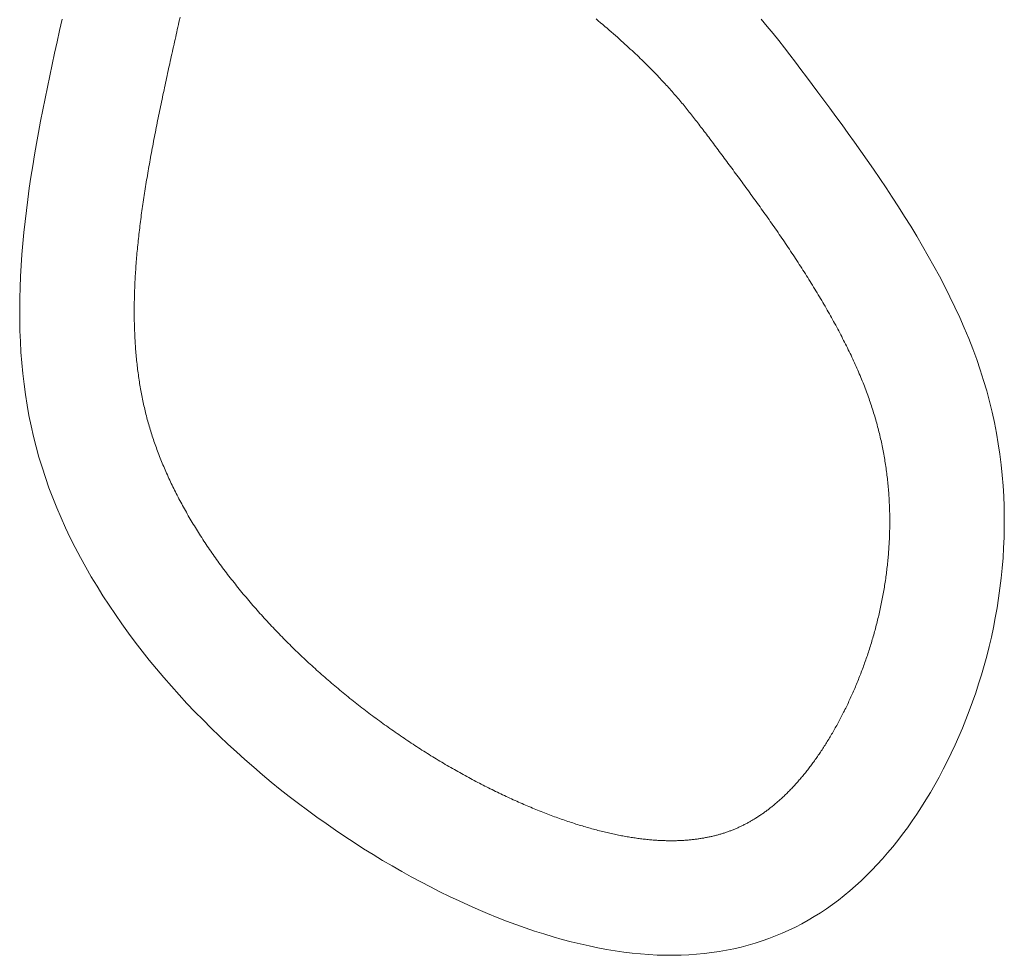
# Model space of a CAD drawing. Units: inches. Extents: x 64 to 1167, y 117 to 939.
# Tile 15 of 56: x 193.497 to 197.794, y 849.033 to 853.116. Entities that reach past the tile are written whole.
import ezdxf

# ---------------------------------------------------------------- set-up
doc = ezdxf.new("R2010")
doc.units = ezdxf.units.IN
doc.header["$MEASUREMENT"] = 0
doc.layers.add('A-FLOR-FIXT', color=8, linetype='Continuous', lineweight=18)

# ---------------------------------------------------------------- blocks, each defined once
blk = doc.blocks.new('FAUCET')
for points in [[(4.0816, 3.6354, 0), (4.1129, 3.6621, 0), (4.144, 3.6879, 0), (4.175, 3.713, 0), (4.2059, 3.7375, 0), (4.2371, 3.7616, 0), (4.2685, 3.7856, 0), (4.3004, 3.8096, 0), (4.3329, 3.8338, 0), (4.366, 3.8585, 0), (4.3999, 3.8837, 0), (4.4345, 3.9094, 0), (4.4699, 3.9356, 0), (4.506, 3.9621, 0), (4.5427, 3.989, 0), (4.5802, 4.0161, 0), (4.6182, 4.0434, 0), (4.6569, 4.0709, 0), (4.6961, 4.0984, 0), (4.7359, 4.126, 0), (4.7762, 4.1535, 0), (4.817, 4.181, 0), (4.8584, 4.2082, 0), (4.9002, 4.2353, 0), (4.9424, 4.2621, 0), (4.985, 4.2886, 0), (5.0281, 4.3147, 0), (5.0715, 4.3404, 0), (5.1152, 4.3655, 0), (5.1593, 4.3901, 0), (5.2036, 4.4141, 0), (5.2483, 4.4374, 0), (5.2931, 4.46, 0), (5.3382, 4.4817, 0), (5.3835, 4.5026, 0), (5.429, 4.5226, 0), (5.4746, 4.5416, 0), (5.5203, 4.5596, 0), (5.5662, 4.5765, 0), (5.6121, 4.5923, 0), (5.6581, 4.6068, 0), (5.7041, 4.6202, 0), (5.7502, 4.6325, 0), (5.7962, 4.6436, 0), (5.8423, 4.6537, 0), (5.8883, 4.6626, 0), (5.9343, 4.6705, 0), (5.9802, 4.6773, 0), (6.0261, 4.6831, 0), (6.0718, 4.6878, 0), (6.1175, 4.6916, 0), (6.163, 4.6944, 0), (6.2084, 4.6962, 0), (6.2536, 4.697, 0), (6.2986, 4.697, 0), (6.3435, 4.696, 0), (6.3882, 4.6942, 0), (6.4326, 4.6915, 0), (6.4768, 4.6879, 0), (6.5207, 4.6835, 0), (6.5644, 4.6782, 0), (6.6078, 4.6722, 0), (6.6509, 4.6654, 0), (6.6936, 4.6578, 0), (6.736, 4.6495, 0), (6.7781, 4.6405, 0), (6.8198, 4.6308, 0), (6.8611, 4.6203, 0), (6.902, 4.6092, 0), (6.9425, 4.5975, 0), (6.9825, 4.5851, 0), (7.0221, 4.5721, 0), (7.0612, 4.5585, 0), (7.0999, 4.5443, 0), (7.138, 4.5295, 0), (7.1756, 4.5143, 0), (7.2127, 4.4985, 0), (7.2492, 4.4821, 0), (7.2852, 4.4653, 0), (7.3206, 4.4481, 0), (7.3553, 4.4303, 0), (7.3895, 4.4122, 0), (7.423, 4.3936, 0), (7.4559, 4.3746, 0), (7.4881, 4.3553, 0), (7.5196, 4.3356, 0), (7.5504, 4.3155, 0), (7.5806, 4.2951, 0), (7.61, 4.2744, 0), (7.6387, 4.2533, 0), (7.6666, 4.2319, 0), (7.6939, 4.2101, 0), (7.7205, 4.188, 0), (7.7463, 4.1655, 0), (7.7714, 4.1426, 0), (7.7957, 4.1195, 0), (7.8193, 4.0959, 0), (7.8422, 4.072, 0), (7.8643, 4.0478, 0), (7.8857, 4.0231, 0), (7.9064, 3.9982, 0), (7.9262, 3.9728, 0), (7.9454, 3.9471, 0), (7.9637, 3.921, 0), (7.9813, 3.8946, 0), (7.9981, 3.8678, 0), (8.0142, 3.8406, 0), (8.0294, 3.8131, 0), (8.0439, 3.7852, 0), (8.0576, 3.7569, 0), (8.0705, 3.7282, 0), (8.0827, 3.6991, 0), (8.094, 3.6697, 0), (8.1045, 3.6399, 0), (8.1142, 3.6097, 0), (8.1231, 3.5791, 0), (8.1312, 3.5482, 0), (8.1385, 3.5168, 0), (8.145, 3.4851, 0), (8.1507, 3.453, 0), (8.1555, 3.4204, 0), (8.1595, 3.3875, 0), (8.1626, 3.3542, 0), (8.165, 3.3205, 0), (8.1665, 3.2864, 0), (8.1671, 3.252, 0), (8.1669, 3.2171, 0), (8.1659, 3.1818, 0), (8.164, 3.1461, 0), (8.1612, 3.11, 0), (8.1576, 3.0735, 0), (8.1531, 3.0366, 0), (8.1477, 2.9992, 0), (8.1415, 2.9615, 0), (8.1344, 2.9234, 0), (8.1264, 2.8849, 0), (8.1176, 2.846, 0), (8.108, 2.8068, 0), (8.0975, 2.7673, 0), (8.0862, 2.7275, 0), (8.074, 2.6874, 0), (8.0611, 2.647, 0), (8.0474, 2.6065, 0), (8.0329, 2.5657, 0), (8.0176, 2.5247, 0), (8.0016, 2.4835, 0), (7.9848, 2.4422, 0), (7.9672, 2.4008, 0), (7.9489, 2.3592, 0), (7.9299, 2.3176, 0), (7.9102, 2.2759, 0), (7.8898, 2.2341, 0), (7.8686, 2.1924, 0), (7.8468, 2.1506, 0), (7.8243, 2.1088, 0), (7.8011, 2.0671, 0), (7.7772, 2.0254, 0), (7.7527, 1.9838, 0), (7.7276, 1.9423, 0), (7.7018, 1.9009, 0), (7.6754, 1.8597, 0), (7.6484, 1.8186, 0), (7.6207, 1.7777, 0), (7.5925, 1.737, 0), (7.5637, 1.6965, 0), (7.5343, 1.6563, 0), (7.5043, 1.6163, 0), (7.4738, 1.5766, 0), (7.4428, 1.5372, 0), (7.4112, 1.4981, 0), (7.379, 1.4594, 0), (7.3464, 1.4211, 0), (7.3132, 1.3831, 0), (7.2795, 1.3456, 0), (7.2453, 1.3085, 0), (7.2107, 1.2718, 0), (7.1755, 1.2356, 0), (7.1399, 1.1999, 0), (7.1039, 1.1647, 0), (7.0674, 1.13, 0), (7.0305, 1.0959, 0), (6.9931, 1.0624, 0), (6.9553, 1.0294, 0), (6.9171, 0.9971, 0), (6.8785, 0.9654, 0), (6.8396, 0.9344, 0), (6.8002, 0.904, 0), (6.7605, 0.8744, 0), (6.7204, 0.8455, 0), (6.6799, 0.8173, 0), (6.6391, 0.7898, 0), (6.598, 0.7632, 0), (6.5566, 0.7373, 0), (6.5148, 0.7123, 0), (6.4727, 0.6881, 0), (6.4304, 0.6648, 0), (6.3877, 0.6424, 0), (6.3448, 0.6208, 0), (6.3016, 0.6002, 0), (6.2581, 0.5806, 0), (6.2144, 0.5619, 0), (6.1705, 0.5442, 0), (6.1263, 0.5275, 0), (6.0819, 0.5119, 0), (6.0373, 0.4973, 0), (5.9925, 0.4837, 0), (5.9475, 0.4713, 0), (5.9023, 0.4599, 0), (5.8569, 0.4497, 0), (5.8114, 0.4404, 0), (5.7657, 0.4322, 0), (5.7198, 0.425, 0), (5.6737, 0.4187, 0), (5.6275, 0.4134, 0), (5.5811, 0.409, 0), (5.5345, 0.4055, 0), (5.4878, 0.4029, 0), (5.441, 0.401, 0), (5.394, 0.4, 0), (5.3468, 0.3998, 0), (5.2995, 0.4004, 0), (5.2521, 0.4017, 0), (5.2045, 0.4036, 0), (5.1568, 0.4063, 0), (5.109, 0.4096, 0), (5.0611, 0.4136, 0), (5.013, 0.4182, 0), (4.9648, 0.4233, 0), (4.9165, 0.429, 0), (4.8681, 0.4352, 0), (4.8196, 0.4419, 0), (4.771, 0.4491, 0), (4.7222, 0.4568, 0), (4.6734, 0.4648, 0), (4.6245, 0.4733, 0), (4.5755, 0.4822, 0), (4.5264, 0.4913, 0), (4.4772, 0.5008, 0), (4.428, 0.5106, 0), (4.3786, 0.5207, 0), (4.3292, 0.531, 0), (4.2798, 0.5415, 0), (4.2302, 0.5522, 0), (4.1806, 0.5631, 0), (4.131, 0.5741, 0), (4.0812, 0.5853, 0)], [(4.0798, 2.9151, 0), (4.0883, 2.9251, 0), (4.0967, 2.935, 0), (4.1049, 2.9447, 0), (4.1131, 2.9542, 0), (4.1212, 2.9636, 0), (4.1292, 2.9729, 0), (4.1371, 2.9819, 0), (4.145, 2.9909, 0), (4.1527, 2.9996, 0), (4.1603, 3.0083, 0), (4.1679, 3.0168, 0), (4.1754, 3.0251, 0), (4.1828, 3.0333, 0), (4.1901, 3.0414, 0), (4.1973, 3.0493, 0), (4.2045, 3.0572, 0), (4.2116, 3.0648, 0), (4.2186, 3.0724, 0), (4.2256, 3.0798, 0), (4.2324, 3.0871, 0), (4.2392, 3.0943, 0), (4.246, 3.1013, 0), (4.2526, 3.1083, 0), (4.2592, 3.1151, 0), (4.2658, 3.1219, 0), (4.2722, 3.1285, 0), (4.2786, 3.135, 0), (4.285, 3.1414, 0), (4.2913, 3.1477, 0), (4.2975, 3.1539, 0), (4.3037, 3.16, 0), (4.3098, 3.166, 0), (4.3159, 3.1719, 0), (4.3219, 3.1777, 0), (4.3279, 3.1835, 0), (4.3338, 3.1891, 0), (4.3397, 3.1947, 0), (4.3456, 3.2002, 0), (4.3514, 3.2057, 0), (4.3572, 3.211, 0), (4.3629, 3.2164, 0), (4.3687, 3.2216, 0), (4.3744, 3.2268, 0), (4.3801, 3.2319, 0), (4.3857, 3.237, 0), (4.3914, 3.242, 0), (4.397, 3.247, 0), (4.4026, 3.252, 0), (4.4082, 3.2569, 0), (4.4138, 3.2617, 0), (4.4194, 3.2665, 0), (4.425, 3.2713, 0), (4.4306, 3.2761, 0), (4.4362, 3.2808, 0), (4.4418, 3.2855, 0), (4.4474, 3.2902, 0), (4.453, 3.2948, 0), (4.4587, 3.2995, 0), (4.4643, 3.3041, 0), (4.47, 3.3087, 0), (4.4756, 3.3133, 0), (4.4813, 3.3179, 0), (4.4871, 3.3224, 0), (4.4928, 3.327, 0), (4.4986, 3.3316, 0), (4.5044, 3.3362, 0), (4.5103, 3.3408, 0), (4.5161, 3.3454, 0), (4.5221, 3.35, 0), (4.528, 3.3546, 0), (4.534, 3.3592, 0), (4.5401, 3.3639, 0), (4.5462, 3.3685, 0), (4.5523, 3.3732, 0), (4.5585, 3.378, 0), (4.5648, 3.3827, 0), (4.5711, 3.3875, 0), (4.5775, 3.3923, 0), (4.5839, 3.3972, 0), (4.5905, 3.4021, 0), (4.597, 3.407, 0), (4.6037, 3.412, 0), (4.6104, 3.417, 0), (4.6172, 3.4221, 0), (4.624, 3.4272, 0), (4.6309, 3.4324, 0), (4.6379, 3.4376, 0), (4.6448, 3.4428, 0), (4.6519, 3.448, 0), (4.659, 3.4533, 0), (4.6661, 3.4586, 0), (4.6733, 3.464, 0), (4.6805, 3.4694, 0), (4.6877, 3.4748, 0), (4.695, 3.4802, 0), (4.7024, 3.4856, 0), (4.7097, 3.4911, 0), (4.7171, 3.4966, 0), (4.7246, 3.5021, 0), (4.732, 3.5076, 0), (4.7395, 3.5132, 0), (4.747, 3.5187, 0), (4.7546, 3.5243, 0), (4.7621, 3.5299, 0), (4.7697, 3.5355, 0), (4.7773, 3.541, 0), (4.7849, 3.5466, 0), (4.7926, 3.5523, 0), (4.8002, 3.5579, 0), (4.8079, 3.5635, 0), (4.8156, 3.5691, 0), (4.8232, 3.5747, 0), (4.8309, 3.5803, 0), (4.8386, 3.5859, 0), (4.8464, 3.5915, 0), (4.8541, 3.5972, 0), (4.8619, 3.6028, 0), (4.8696, 3.6084, 0), (4.8774, 3.614, 0), (4.8852, 3.6196, 0), (4.8931, 3.6253, 0), (4.9009, 3.6309, 0), (4.9088, 3.6365, 0), (4.9167, 3.6421, 0), (4.9246, 3.6478, 0), (4.9325, 3.6534, 0), (4.9404, 3.659, 0), (4.9484, 3.6646, 0), (4.9563, 3.6702, 0), (4.9643, 3.6758, 0), (4.9723, 3.6814, 0), (4.9803, 3.687, 0), (4.9883, 3.6926, 0), (4.9964, 3.6982, 0), (5.0044, 3.7038, 0), (5.0125, 3.7094, 0), (5.0206, 3.7149, 0), (5.0286, 3.7205, 0), (5.0367, 3.726, 0), (5.0449, 3.7316, 0), (5.053, 3.7371, 0), (5.0611, 3.7426, 0), (5.0693, 3.7481, 0), (5.0774, 3.7536, 0), (5.0856, 3.7591, 0), (5.0938, 3.7645, 0), (5.102, 3.77, 0), (5.1102, 3.7754, 0), (5.1184, 3.7808, 0), (5.1266, 3.7862, 0), (5.1349, 3.7916, 0), (5.1431, 3.797, 0), (5.1514, 3.8023, 0), (5.1596, 3.8077, 0), (5.1679, 3.813, 0), (5.1762, 3.8183, 0), (5.1844, 3.8235, 0), (5.1927, 3.8288, 0), (5.201, 3.834, 0), (5.2093, 3.8393, 0), (5.2176, 3.8444, 0), (5.2259, 3.8496, 0), (5.2342, 3.8548, 0), (5.2425, 3.8599, 0), (5.2509, 3.865, 0), (5.2592, 3.8701, 0), (5.2675, 3.8751, 0), (5.2758, 3.8801, 0), (5.2841, 3.8851, 0), (5.2925, 3.8901, 0), (5.3008, 3.8951, 0), (5.3091, 3.9, 0), (5.3174, 3.9049, 0), (5.3258, 3.9097, 0), (5.3341, 3.9146, 0), (5.3424, 3.9194, 0), (5.3507, 3.9241, 0), (5.359, 3.9289, 0), (5.3673, 3.9336, 0), (5.3757, 3.9382, 0), (5.384, 3.9429, 0), (5.3923, 3.9475, 0), (5.4005, 3.9521, 0), (5.4088, 3.9566, 0), (5.4171, 3.9611, 0), (5.4254, 3.9656, 0), (5.4337, 3.97, 0), (5.4419, 3.9744, 0), (5.4502, 3.9788, 0), (5.4584, 3.9831, 0), (5.4667, 3.9874, 0), (5.4749, 3.9916, 0), (5.4831, 3.9959, 0), (5.4913, 4, 0), (5.4995, 4.0042, 0), (5.5077, 4.0082, 0), (5.5159, 4.0123, 0), (5.5241, 4.0163, 0), (5.5322, 4.0203, 0), (5.5403, 4.0242, 0), (5.5485, 4.028, 0), (5.5566, 4.0319, 0), (5.5647, 4.0357, 0), (5.5728, 4.0394, 0), (5.5808, 4.0431, 0), (5.5889, 4.0467, 0), (5.5969, 4.0503, 0), (5.6049, 4.0539, 0), (5.6129, 4.0574, 0), (5.6209, 4.0608, 0), (5.6288, 4.0642, 0), (5.6367, 4.0676, 0), (5.6446, 4.0708, 0), (5.6525, 4.0741, 0), (5.6604, 4.0773, 0), (5.6682, 4.0804, 0), (5.676, 4.0835, 0), (5.6838, 4.0866, 0), (5.6916, 4.0896, 0), (5.6994, 4.0926, 0), (5.7072, 4.0955, 0), (5.7149, 4.0983, 0), (5.7226, 4.1012, 0), (5.7304, 4.1039, 0), (5.7381, 4.1067, 0), (5.7457, 4.1093, 0), (5.7534, 4.112, 0), (5.7611, 4.1146, 0), (5.7687, 4.1171, 0), (5.7764, 4.1196, 0), (5.784, 4.1221, 0), (5.7916, 4.1245, 0), (5.7992, 4.1269, 0), (5.8069, 4.1292, 0), (5.8144, 4.1315, 0), (5.822, 4.1337, 0), (5.8296, 4.1359, 0), (5.8372, 4.1381, 0), (5.8448, 4.1402, 0), (5.8523, 4.1422, 0), (5.8599, 4.1443, 0), (5.8674, 4.1462, 0), (5.875, 4.1482, 0), (5.8825, 4.1501, 0), (5.89, 4.1519, 0), (5.8976, 4.1538, 0), (5.9051, 4.1555, 0), (5.9126, 4.1573, 0), (5.9202, 4.159, 0), (5.9277, 4.1606, 0), (5.9352, 4.1623, 0), (5.9428, 4.1638, 0), (5.9503, 4.1654, 0), (5.9578, 4.1669, 0), (5.9654, 4.1683, 0), (5.9729, 4.1698, 0), (5.9804, 4.1712, 0), (5.988, 4.1725, 0), (5.9955, 4.1738, 0), (6.0031, 4.1751, 0), (6.0106, 4.1763, 0), (6.0182, 4.1775, 0), (6.0257, 4.1787, 0), (6.0333, 4.1798, 0), (6.0409, 4.1809, 0), (6.0485, 4.182, 0), (6.056, 4.183, 0), (6.0636, 4.184, 0), (6.0712, 4.1849, 0), (6.0788, 4.1858, 0), (6.0864, 4.1867, 0), (6.094, 4.1875, 0), (6.1016, 4.1883, 0), (6.1092, 4.1891, 0), (6.1168, 4.1898, 0), (6.1244, 4.1905, 0), (6.132, 4.1912, 0), (6.1396, 4.1918, 0), (6.1472, 4.1924, 0), (6.1548, 4.193, 0), (6.1624, 4.1935, 0), (6.17, 4.194, 0), (6.1776, 4.1944, 0), (6.1852, 4.1948, 0), (6.1928, 4.1952, 0), (6.2004, 4.1956, 0), (6.208, 4.1959, 0), (6.2155, 4.1961, 0), (6.2231, 4.1964, 0), (6.2307, 4.1966, 0), (6.2383, 4.1968, 0), (6.2459, 4.1969, 0), (6.2534, 4.197, 0), (6.261, 4.1971, 0), (6.2686, 4.1971, 0), (6.2761, 4.1971, 0), (6.2837, 4.1971, 0), (6.2913, 4.197, 0), (6.2988, 4.1969, 0), (6.3064, 4.1968, 0), (6.3139, 4.1967, 0), (6.3215, 4.1965, 0), (6.329, 4.1962, 0), (6.3365, 4.196, 0), (6.3441, 4.1957, 0), (6.3516, 4.1954, 0), (6.3591, 4.195, 0), (6.3666, 4.1946, 0), (6.3741, 4.1942, 0), (6.3817, 4.1937, 0), (6.3892, 4.1933, 0), (6.3967, 4.1927, 0), (6.4042, 4.1922, 0), (6.4116, 4.1916, 0), (6.4191, 4.191, 0), (6.4266, 4.1904, 0), (6.4341, 4.1897, 0), (6.4415, 4.189, 0), (6.449, 4.1883, 0), (6.4564, 4.1875, 0), (6.4639, 4.1867, 0), (6.4713, 4.1859, 0), (6.4788, 4.185, 0), (6.4862, 4.1841, 0), (6.4936, 4.1832, 0), (6.501, 4.1823, 0), (6.5084, 4.1813, 0), (6.5158, 4.1803, 0), (6.5232, 4.1793, 0), (6.5306, 4.1782, 0), (6.5379, 4.1771, 0), (6.5453, 4.176, 0), (6.5527, 4.1748, 0), (6.56, 4.1736, 0), (6.5673, 4.1724, 0), (6.5747, 4.1712, 0), (6.582, 4.1699, 0), (6.5893, 4.1686, 0), (6.5966, 4.1673, 0), (6.6039, 4.1659, 0), (6.6112, 4.1645, 0), (6.6185, 4.1631, 0), (6.6257, 4.1616, 0), (6.633, 4.1602, 0), (6.6402, 4.1587, 0), (6.6474, 4.1571, 0), (6.6546, 4.1556, 0), (6.6618, 4.154, 0), (6.669, 4.1524, 0), (6.6762, 4.1507, 0), (6.6834, 4.1491, 0), (6.6905, 4.1474, 0), (6.6977, 4.1457, 0), (6.7048, 4.1439, 0), (6.7119, 4.1421, 0), (6.719, 4.1403, 0), (6.7261, 4.1385, 0), (6.7332, 4.1367, 0), (6.7403, 4.1348, 0), (6.7473, 4.1329, 0), (6.7543, 4.131, 0), (6.7613, 4.129, 0), (6.7683, 4.1271, 0), (6.7753, 4.1251, 0), (6.7823, 4.123, 0), (6.7893, 4.121, 0), (6.7962, 4.1189, 0), (6.8031, 4.1168, 0), (6.81, 4.1147, 0), (6.8169, 4.1126, 0), (6.8238, 4.1104, 0), (6.8307, 4.1082, 0), (6.8375, 4.106, 0), (6.8443, 4.1038, 0), (6.8511, 4.1016, 0), (6.8579, 4.0993, 0), (6.8647, 4.097, 0), (6.8714, 4.0947, 0), (6.8782, 4.0924, 0), (6.8849, 4.09, 0), (6.8916, 4.0876, 0), (6.8982, 4.0852, 0), (6.9049, 4.0828, 0), (6.9115, 4.0804, 0), (6.9181, 4.0779, 0), (6.9247, 4.0754, 0), (6.9313, 4.0729, 0), (6.9379, 4.0704, 0), (6.9444, 4.0679, 0), (6.9509, 4.0653, 0), (6.9574, 4.0628, 0), (6.9639, 4.0602, 0), (6.9703, 4.0576, 0), (6.9767, 4.0549, 0), (6.9831, 4.0523, 0), (6.9895, 4.0496, 0), (6.9959, 4.047, 0), (7.0022, 4.0443, 0), (7.0085, 4.0415, 0), (7.0148, 4.0388, 0), (7.0211, 4.0361, 0), (7.0273, 4.0333, 0), (7.0335, 4.0305, 0), (7.0397, 4.0277, 0), (7.0459, 4.0249, 0), (7.052, 4.0221, 0), (7.0582, 4.0192, 0), (7.0642, 4.0164, 0), (7.0703, 4.0135, 0), (7.0764, 4.0106, 0), (7.0824, 4.0077, 0), (7.0884, 4.0048, 0), (7.0943, 4.0018, 0), (7.1003, 3.9989, 0), (7.1062, 3.9959, 0), (7.1121, 3.9929, 0), (7.1179, 3.99, 0), (7.1238, 3.987, 0), (7.1296, 3.9839, 0), (7.1353, 3.9809, 0), (7.1411, 3.9779, 0), (7.1468, 3.9748, 0), (7.1525, 3.9717, 0), (7.1582, 3.9687, 0), (7.1638, 3.9656, 0), (7.1694, 3.9625, 0), (7.175, 3.9593, 0), (7.1805, 3.9562, 0), (7.186, 3.9531, 0), (7.1915, 3.9499, 0), (7.197, 3.9468, 0), (7.2024, 3.9436, 0), (7.2078, 3.9404, 0), (7.2131, 3.9372, 0), (7.2185, 3.934, 0), (7.2238, 3.9308, 0), (7.229, 3.9276, 0), (7.2343, 3.9244, 0), (7.2395, 3.9211, 0), (7.2447, 3.9179, 0), (7.2498, 3.9146, 0), (7.2549, 3.9114, 0), (7.26, 3.9081, 0), (7.265, 3.9048, 0), (7.27, 3.9015, 0), (7.2749, 3.8983, 0), (7.2798, 3.895, 0), (7.2847, 3.8917, 0), (7.2895, 3.8884, 0), (7.2943, 3.8851, 0), (7.2991, 3.8819, 0), (7.3038, 3.8786, 0), (7.3085, 3.8753, 0), (7.3131, 3.872, 0), (7.3177, 3.8687, 0), (7.3223, 3.8654, 0), (7.3268, 3.8621, 0), (7.3313, 3.8588, 0), (7.3357, 3.8555, 0), (7.3401, 3.8522, 0), (7.3445, 3.8489, 0), (7.3488, 3.8456, 0), (7.3531, 3.8423, 0), (7.3574, 3.839, 0), (7.3616, 3.8357, 0), (7.3658, 3.8324, 0), (7.37, 3.8291, 0), (7.3741, 3.8258, 0), (7.3782, 3.8224, 0), (7.3822, 3.8191, 0), (7.3862, 3.8158, 0), (7.3902, 3.8125, 0), (7.3941, 3.8092, 0), (7.398, 3.8059, 0), (7.4019, 3.8025, 0), (7.4057, 3.7992, 0), (7.4095, 3.7959, 0), (7.4133, 3.7926, 0), (7.417, 3.7892, 0), (7.4207, 3.7859, 0), (7.4243, 3.7826, 0), (7.4279, 3.7793, 0), (7.4315, 3.7759, 0), (7.4351, 3.7726, 0), (7.4386, 3.7693, 0), (7.4421, 3.7659, 0), (7.4455, 3.7626, 0), (7.4489, 3.7593, 0), (7.4523, 3.7559, 0), (7.4557, 3.7526, 0), (7.459, 3.7493, 0), (7.4623, 3.7459, 0), (7.4655, 3.7426, 0), (7.4687, 3.7393, 0), (7.4719, 3.7359, 0), (7.4751, 3.7326, 0), (7.4782, 3.7293, 0), (7.4813, 3.7259, 0), (7.4843, 3.7226, 0), (7.4874, 3.7193, 0), (7.4903, 3.7159, 0), (7.4933, 3.7126, 0), (7.4962, 3.7093, 0), (7.4991, 3.7059, 0), (7.502, 3.7026, 0), (7.5048, 3.6992, 0), (7.5076, 3.6959, 0), (7.5104, 3.6926, 0), (7.5132, 3.6892, 0), (7.5159, 3.6859, 0), (7.5185, 3.6826, 0), (7.5212, 3.6792, 0), (7.5238, 3.6759, 0), (7.5264, 3.6726, 0), (7.529, 3.6692, 0), (7.5315, 3.6659, 0), (7.534, 3.6626, 0), (7.5365, 3.6592, 0), (7.5389, 3.6559, 0), (7.5413, 3.6526, 0), (7.5437, 3.6492, 0), (7.5461, 3.6459, 0), (7.5484, 3.6426, 0), (7.5507, 3.6392, 0), (7.553, 3.6359, 0), (7.5552, 3.6326, 0), (7.5574, 3.6293, 0), (7.5597, 3.6259, 0), (7.5618, 3.6226, 0), (7.564, 3.6193, 0), (7.5661, 3.6159, 0), (7.5682, 3.6126, 0), (7.5703, 3.6092, 0), (7.5724, 3.6059, 0), (7.5744, 3.6026, 0), (7.5764, 3.5992, 0), (7.5784, 3.5959, 0), (7.5803, 3.5925, 0), (7.5823, 3.5891, 0), (7.5842, 3.5858, 0), (7.5861, 3.5824, 0), (7.5879, 3.579, 0), (7.5898, 3.5757, 0), (7.5916, 3.5723, 0), (7.5934, 3.5689, 0), (7.5952, 3.5655, 0), (7.5969, 3.5621, 0), (7.5987, 3.5587, 0), (7.6004, 3.5553, 0), (7.602, 3.5518, 0), (7.6037, 3.5484, 0), (7.6053, 3.545, 0), (7.6069, 3.5415, 0), (7.6085, 3.538, 0), (7.6101, 3.5346, 0), (7.6116, 3.5311, 0), (7.6132, 3.5276, 0), (7.6147, 3.5241, 0), (7.6161, 3.5206, 0), (7.6176, 3.5171, 0), (7.619, 3.5136, 0), (7.6204, 3.51, 0), (7.6218, 3.5065, 0), (7.6232, 3.5029, 0), (7.6245, 3.4994, 0), (7.6259, 3.4958, 0), (7.6272, 3.4922, 0), (7.6284, 3.4886, 0), (7.6297, 3.4849, 0), (7.6309, 3.4813, 0), (7.6322, 3.4777, 0), (7.6333, 3.474, 0), (7.6345, 3.4703, 0), (7.6357, 3.4666, 0), (7.6368, 3.4629, 0), (7.6379, 3.4592, 0), (7.639, 3.4555, 0), (7.6401, 3.4517, 0), (7.6411, 3.4479, 0), (7.6421, 3.4441, 0), (7.6432, 3.4403, 0), (7.6441, 3.4365, 0), (7.6451, 3.4327, 0), (7.646, 3.4288, 0), (7.647, 3.4249, 0), (7.6479, 3.4211, 0), (7.6488, 3.4171, 0), (7.6496, 3.4132, 0), (7.6505, 3.4093, 0), (7.6513, 3.4053, 0), (7.6521, 3.4013, 0), (7.6529, 3.3973, 0), (7.6536, 3.3933, 0), (7.6544, 3.3892, 0), (7.6551, 3.3852, 0), (7.6558, 3.3811, 0), (7.6565, 3.377, 0), (7.6572, 3.3728, 0), (7.6578, 3.3687, 0), (7.6584, 3.3645, 0), (7.6591, 3.3603, 0), (7.6596, 3.3561, 0), (7.6602, 3.3518, 0), (7.6608, 3.3475, 0), (7.6613, 3.3432, 0), (7.6618, 3.3389, 0), (7.6623, 3.3346, 0), (7.6628, 3.3302, 0), (7.6632, 3.3258, 0), (7.6636, 3.3213, 0), (7.664, 3.3169, 0), (7.6644, 3.3124, 0), (7.6647, 3.3079, 0), (7.6651, 3.3033, 0), (7.6654, 3.2988, 0), (7.6657, 3.2941, 0), (7.6659, 3.2895, 0), (7.6661, 3.2849, 0), (7.6663, 3.2802, 0), (7.6665, 3.2755, 0), (7.6667, 3.2707, 0), (7.6668, 3.2659, 0), (7.6669, 3.2611, 0), (7.667, 3.2563, 0), (7.6671, 3.2514, 0), (7.6671, 3.2466, 0), (7.6671, 3.2416, 0), (7.6671, 3.2367, 0), (7.667, 3.2317, 0), (7.6669, 3.2267, 0), (7.6668, 3.2217, 0), (7.6667, 3.2166, 0), (7.6666, 3.2115, 0), (7.6664, 3.2064, 0), (7.6662, 3.2012, 0), (7.6659, 3.1961, 0), (7.6657, 3.1908, 0), (7.6654, 3.1856, 0), (7.665, 3.1803, 0), (7.6647, 3.175, 0), (7.6643, 3.1697, 0), (7.6639, 3.1643, 0), (7.6635, 3.1589, 0), (7.663, 3.1535, 0), (7.6625, 3.148, 0), (7.662, 3.1426, 0), (7.6614, 3.137, 0), (7.6608, 3.1315, 0), (7.6602, 3.1259, 0), (7.6596, 3.1203, 0), (7.6589, 3.1147, 0), (7.6582, 3.109, 0), (7.6574, 3.1033, 0), (7.6567, 3.0975, 0), (7.6559, 3.0918, 0), (7.655, 3.086, 0), (7.6542, 3.0801, 0), (7.6533, 3.0743, 0), (7.6524, 3.0684, 0), (7.6514, 3.0625, 0), (7.6504, 3.0565, 0), (7.6494, 3.0505, 0), (7.6483, 3.0445, 0), (7.6472, 3.0384, 0), (7.6461, 3.0324, 0), (7.645, 3.0262, 0), (7.6438, 3.0201, 0), (7.6425, 3.0139, 0), (7.6413, 3.0077, 0), (7.64, 3.0014, 0), (7.6387, 2.9951, 0), (7.6373, 2.9888, 0), (7.6359, 2.9825, 0), (7.6345, 2.9761, 0), (7.633, 2.9697, 0), (7.6315, 2.9632, 0), (7.63, 2.9567, 0), (7.6284, 2.9502, 0), (7.6268, 2.9437, 0), (7.6252, 2.9371, 0), (7.6235, 2.9305, 0), (7.6218, 2.9238, 0), (7.62, 2.9171, 0), (7.6182, 2.9104, 0), (7.6164, 2.9037, 0), (7.6146, 2.8969, 0), (7.6127, 2.8901, 0), (7.6107, 2.8832, 0), (7.6088, 2.8764, 0), (7.6067, 2.8695, 0), (7.6047, 2.8626, 0), (7.6026, 2.8556, 0), (7.6005, 2.8487, 0), (7.5984, 2.8417, 0), (7.5962, 2.8347, 0), (7.594, 2.8277, 0), (7.5917, 2.8206, 0), (7.5894, 2.8135, 0), (7.5871, 2.8064, 0), (7.5848, 2.7993, 0), (7.5824, 2.7921, 0), (7.58, 2.785, 0), (7.5775, 2.7778, 0), (7.575, 2.7706, 0), (7.5725, 2.7634, 0), (7.5699, 2.7561, 0), (7.5673, 2.7488, 0), (7.5647, 2.7415, 0), (7.562, 2.7342, 0), (7.5593, 2.7269, 0), (7.5566, 2.7196, 0), (7.5538, 2.7122, 0), (7.551, 2.7048, 0), (7.5482, 2.6974, 0), (7.5453, 2.69, 0), (7.5424, 2.6826, 0), (7.5395, 2.6751, 0), (7.5365, 2.6677, 0), (7.5335, 2.6602, 0), (7.5305, 2.6527, 0), (7.5274, 2.6452, 0), (7.5243, 2.6376, 0), (7.5212, 2.6301, 0), (7.518, 2.6225, 0), (7.5148, 2.615, 0), (7.5116, 2.6074, 0), (7.5083, 2.5998, 0), (7.505, 2.5922, 0), (7.5017, 2.5846, 0), (7.4984, 2.5769, 0), (7.495, 2.5693, 0), (7.4915, 2.5616, 0), (7.4881, 2.554, 0), (7.4846, 2.5463, 0), (7.4811, 2.5386, 0), (7.4775, 2.5309, 0), (7.4739, 2.5232, 0), (7.4703, 2.5155, 0), (7.4667, 2.5077, 0), (7.463, 2.5, 0), (7.4593, 2.4923, 0), (7.4555, 2.4845, 0), (7.4518, 2.4767, 0), (7.448, 2.469, 0), (7.4441, 2.4612, 0), (7.4403, 2.4534, 0), (7.4364, 2.4456, 0), (7.4324, 2.4378, 0), (7.4285, 2.43, 0), (7.4245, 2.4222, 0), (7.4205, 2.4144, 0), (7.4164, 2.4066, 0), (7.4123, 2.3987, 0), (7.4082, 2.3909, 0), (7.4041, 2.3831, 0), (7.3999, 2.3753, 0), (7.3957, 2.3674, 0), (7.3915, 2.3596, 0), (7.3872, 2.3517, 0), (7.3829, 2.3439, 0), (7.3786, 2.336, 0), (7.3742, 2.3282, 0), (7.3699, 2.3203, 0), (7.3654, 2.3125, 0), (7.361, 2.3046, 0), (7.3565, 2.2968, 0), (7.352, 2.2889, 0), (7.3475, 2.2811, 0), (7.3429, 2.2732, 0), (7.3383, 2.2653, 0), (7.3337, 2.2575, 0), (7.3291, 2.2496, 0), (7.3244, 2.2418, 0), (7.3197, 2.2339, 0), (7.315, 2.2261, 0), (7.3102, 2.2182, 0), (7.3054, 2.2104, 0), (7.3006, 2.2026, 0), (7.2958, 2.1947, 0), (7.2909, 2.1869, 0), (7.286, 2.1791, 0), (7.2811, 2.1712, 0), (7.2762, 2.1634, 0), (7.2712, 2.1556, 0), (7.2662, 2.1478, 0), (7.2612, 2.1399, 0), (7.2561, 2.1321, 0), (7.251, 2.1243, 0), (7.2459, 2.1165, 0), (7.2408, 2.1087, 0), (7.2356, 2.1009, 0), (7.2304, 2.0932, 0), (7.2252, 2.0854, 0), (7.22, 2.0776, 0), (7.2147, 2.0699, 0), (7.2094, 2.0621, 0), (7.2041, 2.0543, 0), (7.1988, 2.0466, 0), (7.1934, 2.0389, 0), (7.188, 2.0311, 0), (7.1826, 2.0234, 0), (7.1772, 2.0157, 0), (7.1717, 2.008, 0), (7.1662, 2.0003, 0), (7.1607, 1.9926, 0), (7.1552, 1.985, 0), (7.1496, 1.9773, 0), (7.144, 1.9697, 0), (7.1384, 1.962, 0), (7.1328, 1.9544, 0), (7.1272, 1.9468, 0), (7.1215, 1.9391, 0), (7.1158, 1.9316, 0), (7.1101, 1.924, 0), (7.1043, 1.9164, 0), (7.0986, 1.9088, 0), (7.0928, 1.9013, 0), (7.087, 1.8937, 0), (7.0811, 1.8862, 0), (7.0753, 1.8787, 0), (7.0694, 1.8712, 0), (7.0635, 1.8637, 0), (7.0576, 1.8562, 0), (7.0516, 1.8488, 0), (7.0457, 1.8413, 0), (7.0397, 1.8339, 0), (7.0337, 1.8265, 0), (7.0276, 1.8191, 0), (7.0216, 1.8117, 0), (7.0155, 1.8043, 0), (7.0094, 1.797, 0), (7.0033, 1.7896, 0), (6.9972, 1.7823, 0), (6.991, 1.775, 0), (6.9849, 1.7677, 0), (6.9787, 1.7604, 0), (6.9725, 1.7532, 0), (6.9662, 1.746, 0), (6.96, 1.7387, 0), (6.9537, 1.7315, 0), (6.9474, 1.7244, 0), (6.9411, 1.7172, 0), (6.9348, 1.71, 0), (6.9284, 1.7029, 0), (6.9221, 1.6958, 0), (6.9157, 1.6887, 0), (6.9093, 1.6817, 0), (6.9029, 1.6746, 0), (6.8964, 1.6676, 0), (6.89, 1.6606, 0), (6.8835, 1.6536, 0), (6.877, 1.6466, 0), (6.8705, 1.6397, 0), (6.864, 1.6328, 0), (6.8574, 1.6259, 0), (6.8509, 1.619, 0), (6.8443, 1.6121, 0), (6.8377, 1.6053, 0), (6.8311, 1.5985, 0), (6.8244, 1.5917, 0), (6.8178, 1.5849, 0), (6.8111, 1.5782, 0), (6.8045, 1.5715, 0), (6.7978, 1.5648, 0), (6.7911, 1.5581, 0), (6.7843, 1.5515, 0), (6.7776, 1.5448, 0), (6.7708, 1.5382, 0), (6.7641, 1.5317, 0), (6.7573, 1.5251, 0), (6.7505, 1.5186, 0), (6.7437, 1.5121, 0), (6.7368, 1.5056, 0), (6.73, 1.4992, 0), (6.7231, 1.4927, 0), (6.7163, 1.4864, 0), (6.7094, 1.48, 0), (6.7025, 1.4736, 0), (6.6956, 1.4673, 0), (6.6887, 1.461, 0), (6.6817, 1.4548, 0), (6.6748, 1.4485, 0), (6.6678, 1.4423, 0), (6.6608, 1.4361, 0), (6.6539, 1.43, 0), (6.6469, 1.4238, 0), (6.6398, 1.4177, 0), (6.6328, 1.4117, 0), (6.6258, 1.4056, 0), (6.6187, 1.3996, 0), (6.6117, 1.3936, 0), (6.6046, 1.3877, 0), (6.5975, 1.3818, 0), (6.5905, 1.3759, 0), (6.5834, 1.37, 0), (6.5763, 1.3642, 0), (6.5691, 1.3584, 0), (6.562, 1.3526, 0), (6.5549, 1.3468, 0), (6.5477, 1.3411, 0), (6.5406, 1.3354, 0), (6.5334, 1.3298, 0), (6.5262, 1.3242, 0), (6.519, 1.3186, 0), (6.5118, 1.313, 0), (6.5046, 1.3075, 0), (6.4974, 1.302, 0), (6.4902, 1.2965, 0), (6.483, 1.2911, 0), (6.4757, 1.2857, 0), (6.4685, 1.2803, 0), (6.4612, 1.275, 0), (6.454, 1.2697, 0), (6.4467, 1.2645, 0), (6.4394, 1.2592, 0), (6.4322, 1.254, 0), (6.4249, 1.2489, 0), (6.4176, 1.2438, 0), (6.4103, 1.2387, 0), (6.403, 1.2336, 0), (6.3956, 1.2286, 0), (6.3883, 1.2236, 0), (6.381, 1.2187, 0), (6.3737, 1.2137, 0), (6.3663, 1.2089, 0), (6.359, 1.204, 0), (6.3517, 1.1992, 0), (6.3443, 1.1944, 0), (6.3369, 1.1897, 0), (6.3296, 1.185, 0), (6.3222, 1.1804, 0), (6.3149, 1.1757, 0), (6.3075, 1.1711, 0), (6.3001, 1.1666, 0), (6.2927, 1.1621, 0), (6.2854, 1.1576, 0), (6.278, 1.1532, 0), (6.2706, 1.1488, 0), (6.2632, 1.1444, 0), (6.2558, 1.1401, 0), (6.2484, 1.1358, 0), (6.241, 1.1315, 0), (6.2336, 1.1273, 0), (6.2262, 1.1232, 0), (6.2188, 1.119, 0), (6.2114, 1.1149, 0), (6.204, 1.1109, 0), (6.1966, 1.1068, 0), (6.1892, 1.1029, 0), (6.1818, 1.0989, 0), (6.1744, 1.095, 0), (6.167, 1.0911, 0), (6.1595, 1.0873, 0), (6.1521, 1.0835, 0), (6.1447, 1.0798, 0), (6.1373, 1.0761, 0), (6.1299, 1.0724, 0), (6.1225, 1.0688, 0), (6.1151, 1.0652, 0), (6.1077, 1.0616, 0), (6.1003, 1.0581, 0), (6.0929, 1.0546, 0), (6.0855, 1.0512, 0), (6.0781, 1.0478, 0), (6.0707, 1.0445, 0), (6.0633, 1.0411, 0), (6.0559, 1.0379, 0), (6.0485, 1.0346, 0), (6.0411, 1.0314, 0), (6.0337, 1.0283, 0), (6.0263, 1.0252, 0), (6.0189, 1.0221, 0), (6.0115, 1.0191, 0), (6.0042, 1.0161, 0), (5.9968, 1.0132, 0), (5.9894, 1.0103, 0), (5.982, 1.0074, 0), (5.9747, 1.0046, 0), (5.9673, 1.0018, 0), (5.96, 0.9991, 0), (5.9526, 0.9964, 0), (5.9453, 0.9937, 0), (5.9379, 0.9911, 0), (5.9306, 0.9886, 0), (5.9233, 0.986, 0), (5.9159, 0.9835, 0), (5.9086, 0.9811, 0), (5.9013, 0.9787, 0), (5.894, 0.9763, 0), (5.8866, 0.974, 0), (5.8793, 0.9717, 0), (5.872, 0.9695, 0), (5.8646, 0.9673, 0), (5.8573, 0.9651, 0), (5.85, 0.963, 0), (5.8427, 0.9609, 0), (5.8353, 0.9589, 0), (5.828, 0.9569, 0), (5.8206, 0.9549, 0), (5.8133, 0.953, 0), (5.8059, 0.9511, 0), (5.7985, 0.9493, 0), (5.7912, 0.9475, 0), (5.7838, 0.9457, 0), (5.7764, 0.9439, 0), (5.769, 0.9422, 0), (5.7616, 0.9406, 0), (5.7541, 0.939, 0), (5.7467, 0.9374, 0), (5.7392, 0.9358, 0), (5.7318, 0.9343, 0), (5.7243, 0.9328, 0), (5.7168, 0.9314, 0), (5.7093, 0.9299, 0), (5.7018, 0.9286, 0), (5.6942, 0.9272, 0), (5.6867, 0.9259, 0), (5.6791, 0.9246, 0), (5.6715, 0.9234, 0), (5.6639, 0.9222, 0), (5.6563, 0.921, 0), (5.6486, 0.9199, 0), (5.6409, 0.9188, 0), (5.6333, 0.9177, 0), (5.6255, 0.9166, 0), (5.6178, 0.9156, 0), (5.61, 0.9146, 0), (5.6023, 0.9137, 0), (5.5944, 0.9128, 0), (5.5866, 0.9119, 0), (5.5787, 0.911, 0), (5.5709, 0.9102, 0), (5.5629, 0.9094, 0), (5.555, 0.9087, 0), (5.547, 0.9079, 0), (5.5391, 0.9072, 0), (5.531, 0.9066, 0), (5.523, 0.9059, 0), (5.515, 0.9053, 0), (5.5069, 0.9048, 0), (5.4988, 0.9042, 0), (5.4907, 0.9037, 0), (5.4825, 0.9033, 0), (5.4744, 0.9028, 0), (5.4662, 0.9024, 0), (5.458, 0.902, 0), (5.4498, 0.9017, 0), (5.4415, 0.9014, 0), (5.4333, 0.9011, 0), (5.425, 0.9008, 0), (5.4167, 0.9006, 0), (5.4083, 0.9004, 0), (5.4, 0.9002, 0), (5.3916, 0.9001, 0), (5.3832, 0.9, 0), (5.3748, 0.8999, 0), (5.3663, 0.8999, 0), (5.3579, 0.8998, 0), (5.3494, 0.8999, 0), (5.3409, 0.8999, 0), (5.3324, 0.9, 0), (5.3238, 0.9001, 0), (5.3152, 0.9002, 0), (5.3067, 0.9004, 0), (5.298, 0.9005, 0), (5.2894, 0.9008, 0), (5.2808, 0.901, 0), (5.2721, 0.9013, 0), (5.2634, 0.9016, 0), (5.2547, 0.9019, 0), (5.2459, 0.9023, 0), (5.2372, 0.9027, 0), (5.2284, 0.9031, 0), (5.2196, 0.9035, 0), (5.2107, 0.904, 0), (5.2019, 0.9045, 0), (5.193, 0.905, 0), (5.1841, 0.9056, 0), (5.1752, 0.9062, 0), (5.1663, 0.9068, 0), (5.1573, 0.9074, 0), (5.1484, 0.9081, 0), (5.1394, 0.9088, 0), (5.1303, 0.9095, 0), (5.1213, 0.9103, 0), (5.1122, 0.911, 0), (5.1032, 0.9118, 0), (5.0941, 0.9127, 0), (5.0849, 0.9135, 0), (5.0758, 0.9144, 0), (5.0666, 0.9153, 0), (5.0575, 0.9163, 0), (5.0483, 0.9172, 0), (5.039, 0.9182, 0), (5.0298, 0.9192, 0), (5.0205, 0.9203, 0), (5.0113, 0.9213, 0), (5.002, 0.9224, 0), (4.9927, 0.9235, 0), (4.9833, 0.9247, 0), (4.974, 0.9258, 0), (4.9646, 0.927, 0), (4.9552, 0.9282, 0), (4.9458, 0.9295, 0), (4.9364, 0.9307, 0), (4.9269, 0.932, 0), (4.9174, 0.9333, 0), (4.908, 0.9347, 0), (4.8984, 0.936, 0), (4.8889, 0.9374, 0), (4.8794, 0.9388, 0), (4.8698, 0.9402, 0), (4.8602, 0.9417, 0), (4.8506, 0.9431, 0), (4.841, 0.9446, 0), (4.8314, 0.9461, 0), (4.8217, 0.9476, 0), (4.8121, 0.9492, 0), (4.8024, 0.9507, 0), (4.7927, 0.9523, 0), (4.783, 0.9539, 0), (4.7732, 0.9556, 0), (4.7635, 0.9572, 0), (4.7537, 0.9589, 0), (4.7439, 0.9606, 0), (4.7341, 0.9623, 0), (4.7243, 0.964, 0), (4.7144, 0.9657, 0), (4.7045, 0.9675, 0), (4.6947, 0.9693, 0), (4.6848, 0.9711, 0), (4.6749, 0.9729, 0), (4.6649, 0.9747, 0), (4.655, 0.9765, 0), (4.645, 0.9784, 0), (4.635, 0.9803, 0), (4.625, 0.9822, 0), (4.615, 0.9841, 0), (4.605, 0.986, 0), (4.5949, 0.988, 0), (4.5849, 0.9899, 0), (4.5748, 0.9919, 0), (4.5647, 0.9939, 0), (4.5546, 0.9959, 0), (4.5444, 0.9979, 0), (4.5343, 0.9999, 0), (4.5241, 1.002, 0), (4.514, 1.004, 0), (4.5038, 1.0061, 0), (4.4936, 1.0082, 0), (4.4833, 1.0103, 0), (4.4731, 1.0124, 0), (4.4628, 1.0145, 0), (4.4526, 1.0167, 0), (4.4423, 1.0188, 0), (4.432, 1.021, 0), (4.4217, 1.0231, 0), (4.4113, 1.0253, 0), (4.401, 1.0275, 0), (4.3906, 1.0297, 0), (4.3802, 1.032, 0), (4.3698, 1.0342, 0), (4.3594, 1.0364, 0), (4.349, 1.0387, 0), (4.3386, 1.0409, 0), (4.3281, 1.0432, 0), (4.3177, 1.0455, 0), (4.3072, 1.0478, 0), (4.2967, 1.05, 0), (4.2862, 1.0524, 0), (4.2756, 1.0547, 0), (4.2651, 1.057, 0), (4.2546, 1.0593, 0), (4.244, 1.0616, 0), (4.2334, 1.064, 0), (4.2228, 1.0663, 0), (4.2122, 1.0687, 0), (4.2016, 1.0711, 0), (4.1909, 1.0734, 0), (4.1803, 1.0758, 0), (4.1696, 1.0782, 0), (4.1589, 1.0806, 0), (4.1482, 1.083, 0), (4.1375, 1.0854, 0), (4.1268, 1.0878, 0), (4.1161, 1.0902, 0), (4.1053, 1.0926, 0), (4.0946, 1.0951, 0), (4.0838, 1.0975, 0), (4.073, 1.0999, 0)]]:
    blk.add_polyline3d(points)

msp = doc.modelspace()

# ---------------------------------------------------------------- block references
at = {"layer": 'A-FLOR-FIXT', "rotation": 270.0000000000299}
msp.add_blockref('FAUCET', (193.0969, 857.2), dxfattribs=at)

doc.saveas('drawing.dxf')
